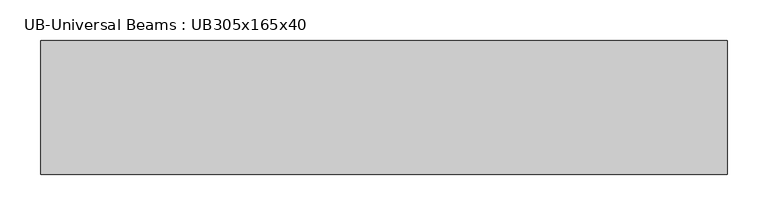
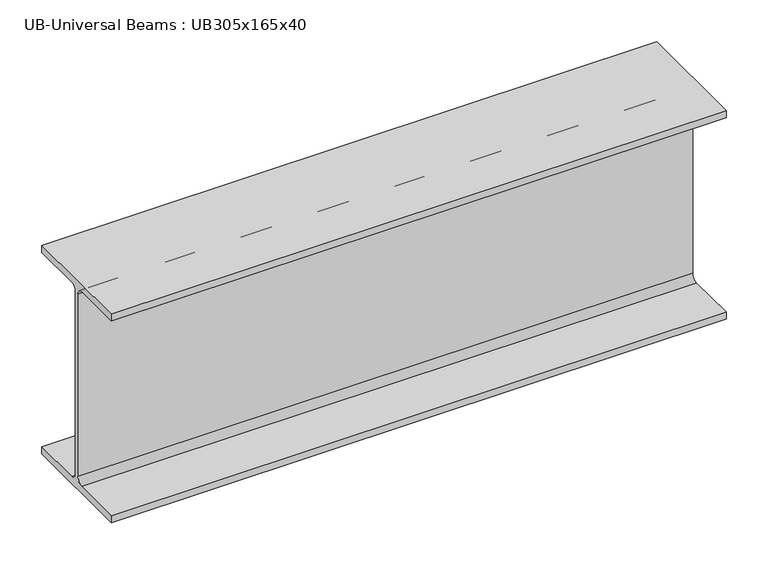
"""IFC4 building model written with IfcOpenShell, lengths in millimetres: beam geometry, UB-Universal Beams : UB305x165x40."""

from ifc_helpers import new_model, si_unit, point, frame, frame_2d, origin, place, context, project, spatial, polyline, circle_curve, trimmed, segment, composite_curve, outline, extrude, source, transform, mapped, element, save


def ub_universal_beams_ub305x165x40_eb09afc0(model_context):
    return source(origin(), model_context, "Body", "SweptSolid", [
        extrude(outline(composite_curve([segment(polyline([(82.5, -141.5), (82.5, -151.7), (-82.5, -151.7), (-82.5, -141.5), (-11.9, -141.5)]), True, "CONTINUOUS"), segment(trimmed(circle_curve(frame_2d((-11.9, -132.6)), 8.9), [point((-11.9, -141.5))], [point((-3.0, -132.6))], True, "CARTESIAN"), True, "CONTINUOUS"), segment(polyline([(-3.0, -132.6), (-3.0, 132.6)]), True, "CONTINUOUS"), segment(trimmed(circle_curve(frame_2d((-11.9, 132.6)), 8.9), [point((-3.0, 132.6))], [point((-11.9, 141.5))], True, "CARTESIAN"), True, "CONTINUOUS"), segment(polyline([(-11.9, 141.5), (-82.5, 141.5), (-82.5, 151.7), (82.5, 151.7), (82.5, 141.5), (11.9, 141.5)]), True, "CONTINUOUS"), segment(trimmed(circle_curve(frame_2d((11.9, 132.6)), 8.9), [point((11.9, 141.5))], [point((3.0, 132.6))], True, "CARTESIAN"), True, "CONTINUOUS"), segment(polyline([(3.0, 132.6), (3.0, -132.6)]), True, "CONTINUOUS"), segment(trimmed(circle_curve(frame_2d((11.9, -132.6)), 8.9), [point((3.0, -132.6))], [point((11.9, -141.5))], True, "CARTESIAN"), True, "CONTINUOUS"), segment(polyline([(11.9, -141.5), (82.5, -141.5)]), True, "CONTINUOUS")], self_intersect=False)), frame((-435.6, 0.0, 0.0), z_axis=(1.0, 0.0, 0.0), x_axis=(0.0, 1.0, 0.0)), (0.0, 0.0, 1.0), 845.4),
    ])


if __name__ == "__main__":
    model = new_model("IFC4")
    model_context = context("Model", 3, world=origin())
    ifc_project = project(units=[si_unit("LENGTHUNIT", "METRE", prefix="MILLI")], contexts=[model_context])
    site = spatial("IfcSite", under=ifc_project)
    building = spatial("IfcBuilding", under=site)
    placement = place(None, origin())
    ub_universal_beams_ub305x165x40_shape = ub_universal_beams_ub305x165x40_eb09afc0(model_context)
    element("IfcBeam", 1, ObjectType="UB-Universal Beams : UB305x165x40", at=placement, inside=building, context=model_context, shape_type="MappedRepresentation", body=[
        mapped(ub_universal_beams_ub305x165x40_shape, transform((0.0, 0.0, 0.0), x_axis=(1.0, 0.0, 0.0), y_axis=(0.0, 1.0, 0.0), z_axis=(0.0, 0.0, 1.0))),
    ])
    save(model, "model.ifc")

# Revit data of these elements
# Type "UB-Universal Beams : UB305x165x40"
#   Section Name Key = "UB305X165X40"
#   Width = 16.5 cm
#   Web Thickness = 0.6 cm
#   Web Fillet = 0.89 cm
#   Warping Constant = 164000.0 cm⁶
#   Torsional Moment of Inertia = 14.70 cm⁴
#   Section Area = 51.3 cm²
#   Plastic Modulus weak axis = 142.0 cm³
#   Plastic Modulus strong axis = 623.0 cm³
#   Nominal Weight = 40.2999 kgf/m
#   Moment of Inertia weak axis = 764.00 cm⁴
#   Moment of Inertia strong axis = 8503.00 cm⁴
#   Height = 30.34 cm
#   Flange Thickness = 1.02 cm
#   Elastic Modulus weak axis = 92.6 cm³
#   Elastic Modulus strong axis = 560.0 cm³
#   Centroid Vertical = 15.17 cm
#   Centroid Horizontal = 8.25 cm
#   Bolt Spacing = 9.0 cm
#   Length [instance default] = 1500 mm
#   Structural Material [instance default] = Metal - Steel 43-275
#   Type Comments = ""
#   Assembly Code = ""
# Element 1 (IfcBeam, "UB-Universal Beams : UB305x165x40")
#   Materials on its faces: "Metal - Steel 43-275"
# Materials
#   "Metal - Steel 43-275": class "Metal", colour RGB 247 247 247, transparency 0, Cost = 0
